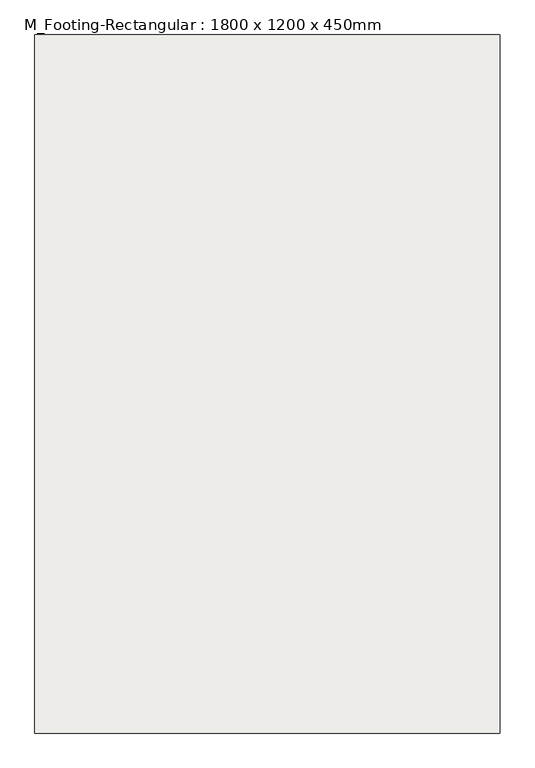
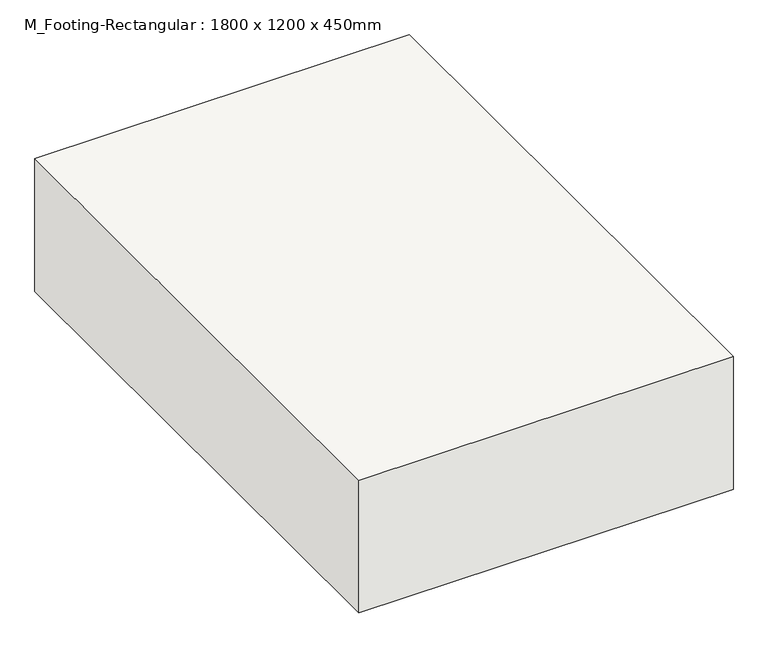
"""IFC4 building model written with IfcOpenShell, lengths in millimetres: slab geometry, M_Footing-Rectangular : 1800 x 1200 x 450mm."""

from ifc_helpers import new_model, si_unit, frame, origin, place, context, project, spatial, polyline, outline, extrude, source, transform, mapped, element, save


def m_footing_rectangular_1800_x_1200_x_450mm_16ba7ea5(model_context):
    return source(origin(), model_context, "Body", "SweptSolid", [
        extrude(outline(polyline([(600.0, 900.0), (600.0, -900.0), (-600.0, -900.0), (-600.0, 900.0), (600.0, 900.0)])), frame((0.0, 0.0, -450.0), z_axis=(0.0, 0.0, 1.0), x_axis=(1.0, 0.0, 0.0)), (0.0, 0.0, 1.0), 450.0),
    ])


if __name__ == "__main__":
    model = new_model("IFC4")
    model_context = context("Model", 3, world=origin())
    ifc_project = project(units=[si_unit("LENGTHUNIT", "METRE", prefix="MILLI")], contexts=[model_context])
    site = spatial("IfcSite", under=ifc_project)
    building = spatial("IfcBuilding", under=site)
    placement = place(None, origin())
    m_footing_rectangular_1800_x_1200_x_450mm_shape = m_footing_rectangular_1800_x_1200_x_450mm_16ba7ea5(model_context)
    element("IfcSlab", 1, ObjectType="M_Footing-Rectangular : 1800 x 1200 x 450mm", at=placement, inside=building, context=model_context, shape_type="MappedRepresentation", body=[
        mapped(m_footing_rectangular_1800_x_1200_x_450mm_shape, transform((0.0, 0.0, 0.0), x_axis=(1.0, 0.0, 0.0), y_axis=(0.0, 1.0, 0.0), z_axis=(0.0, 0.0, 1.0))),
    ])
    save(model, "model.ifc")

# Revit data of these elements
# Type "M_Footing-Rectangular : 1800 x 1200 x 450mm"
#   Width = 1200 mm
#   Length = 1800 mm
#   Foundation Thickness = 450 mm
#   Structural Material [instance default] = Concrete, Cast-in-Place gray
#   Assembly Code = ""
# Element 1 (IfcSlab, "M_Footing-Rectangular : 1800 x 1200 x 450mm")
#   Materials on its faces: "Concrete, Cast-in-Place gray"
# Materials
#   "Concrete, Cast-in-Place gray": class "Concrete", colour RGB 192 192 192, transparency 0, Description = "Cast-in-place concrete", Cost = 0
